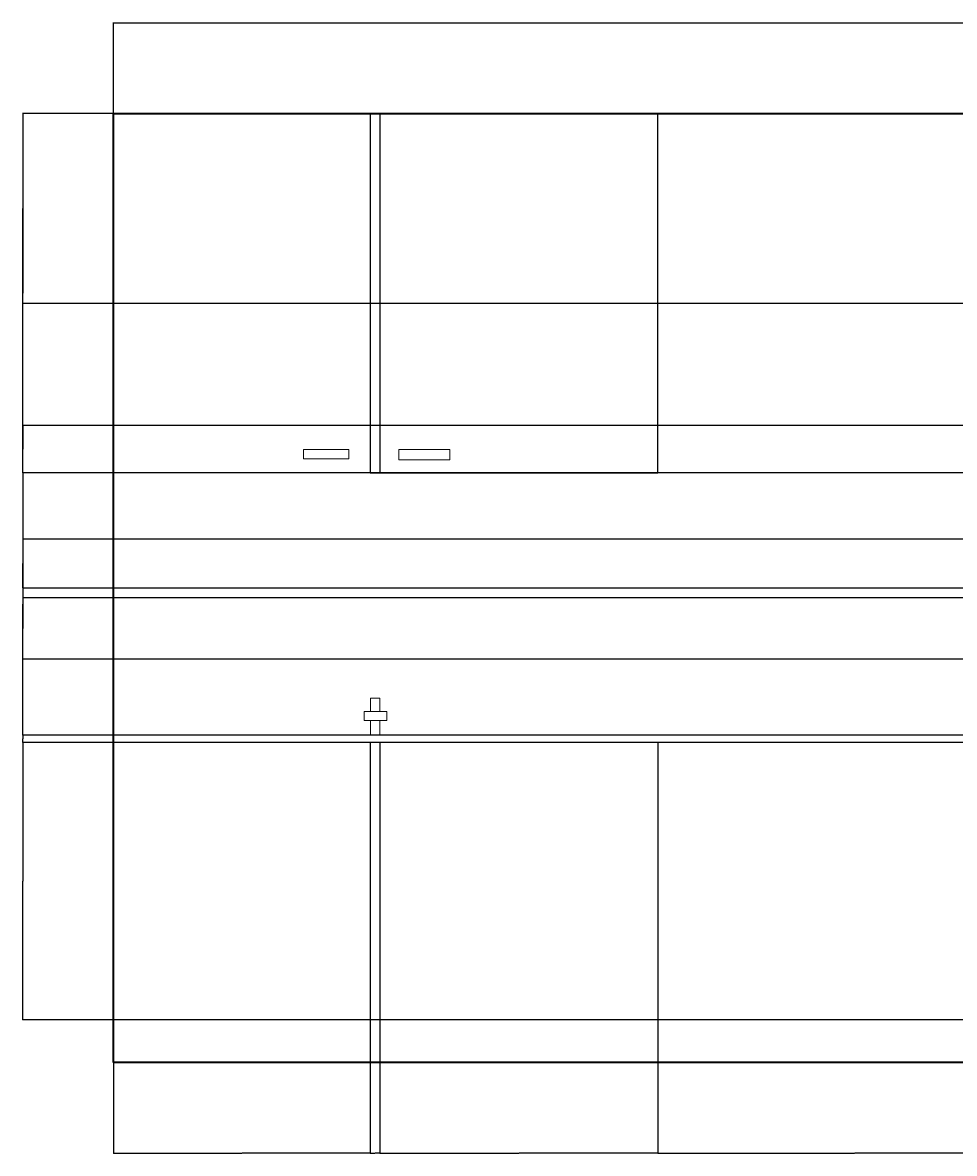
# Model space of a CAD drawing. Units: millimetres. Extents: x 4725 to 8727, y 2935 to 5260.
# Tile 1 of 3: x 4725 to 6642, y 2935 to 5260. Entities that reach past the tile are written whole.
import ezdxf

# ---------------------------------------------------------------- set-up
doc = ezdxf.new("R2010")
doc.units = ezdxf.units.MM
for name, color, linetype, lineweight in [('A-ANNO-DIMS', 2, 'Continuous', 18), ('A-CASE-CTOP', 7, 'Continuous', 25), ('A-CASE-HRDW', 9, 'Continuous', 13), ('A-ELEV', 7, 'Continuous', 35), ('A-FLOR-CASE', 8, 'Continuous', 25), ('A-FLOR-FIXT', 9, 'Continuous', 18)]:
    doc.layers.add(name, color=color, linetype=linetype, lineweight=lineweight)
doc.styles.get("Standard").update_dxf_attribs({"font": 'arial.ttf'})
doc.dimstyles.get("Standard").update_dxf_attribs({"dimtxt": 0.18, "dimasz": 0.18, "dimexe": 0.18, "dimexo": 0.0625, "dimgap": 0.09, "dimtad": 0, "dimtih": 1, "dimtoh": 1, "dimdec": 4, "dimzin": 0, "dimdsep": 46, "dimtxsty": 'Standard', "dimcen": 0.09, "dimadec": 0, "dimazin": 0, "dimtfac": 1, "dimtdec": 4, "dimtofl": 0, "dimtmove": 0, "dimatfit": 3, "dimfxl": 1, "dimtolj": 1, "dimtzin": 0, "dimarcsym": 0})

# ---------------------------------------------------------------- blocks, each defined once
blk = doc.blocks.new('*D7')
at = {"layer": 'A-ANNO-DIMS', "color": 0, "lineweight": -2, "transparency": 16777216}
for p, q in [((4912.4, 3209), (4912.4, 2934.7)), ((5440.1, 3209), (5440.1, 2934.7)), ((4912.5, 2934.8), (5175.9, 2934.8)), ((5440, 2934.8), (5176.6, 2934.8))]:
    blk.add_line(p, q, dxfattribs=at)
at = {"layer": 'A-ANNO-DIMS', "color": 0, "transparency": 16777216}
for points in [[(4912.5, 2934.9), (4912.5, 2934.8), (4912.4, 2934.8)], [(5440, 2934.9), (5440, 2934.8), (5440.1, 2934.8)]]:
    blk.add_solid(points, dxfattribs=at)
at = {"layer": 'Defpoints', "color": 0, "transparency": 16777216}
for p in [(4912.4, 3209), (5440.1, 3209), (5440.1, 2934.8)]:
    blk.add_point(p, dxfattribs=at)
at = {"layer": 'A-ANNO-DIMS', "color": 0, "transparency": 16777216, "insert": (5176.3, 2934.8), "char_height": 0.18, "attachment_point": 5}
blk.add_mtext('\\A1;527.8', dxfattribs=at)
blk = doc.blocks.new('*D8')
at = {"layer": 'A-ANNO-DIMS', "color": 0, "lineweight": -2, "transparency": 16777216}
for p, q in [((5440.1, 3209), (5440.1, 2934.7)), ((5460.1, 3209), (5460.1, 2934.7)), ((5440.3, 2934.8), (5449.9, 2934.8)), ((5460, 2934.8), (5450.4, 2934.8))]:
    blk.add_line(p, q, dxfattribs=at)
at = {"layer": 'A-ANNO-DIMS', "color": 0, "transparency": 16777216}
for points in [[(5440.3, 2934.9), (5440.3, 2934.8), (5440.1, 2934.8)], [(5460, 2934.9), (5460, 2934.8), (5460.1, 2934.8)]]:
    blk.add_solid(points, dxfattribs=at)
at = {"layer": 'Defpoints', "color": 0, "transparency": 16777216}
for p in [(5440.1, 3209), (5460.1, 3209), (5460.1, 2934.8)]:
    blk.add_point(p, dxfattribs=at)
at = {"layer": 'A-ANNO-DIMS', "color": 0, "transparency": 16777216, "insert": (5450.1, 2934.8), "char_height": 0.18, "attachment_point": 5}
blk.add_mtext('\\A1;20', dxfattribs=at)
blk = doc.blocks.new('*D9')
at = {"layer": 'A-ANNO-DIMS', "color": 0, "lineweight": -2, "transparency": 16777216}
for p, q in [((5460.1, 3209), (5460.1, 2934.7)), ((6031.8, 3209), (6031.8, 2934.7)), ((5460.3, 2934.8), (5745.6, 2934.8)), ((6031.6, 2934.8), (5746.4, 2934.8))]:
    blk.add_line(p, q, dxfattribs=at)
at = {"layer": 'A-ANNO-DIMS', "color": 0, "transparency": 16777216}
for points in [[(5460.3, 2934.9), (5460.3, 2934.8), (5460.1, 2934.8)], [(6031.6, 2934.9), (6031.6, 2934.8), (6031.8, 2934.8)]]:
    blk.add_solid(points, dxfattribs=at)
at = {"layer": 'Defpoints', "color": 0, "transparency": 16777216}
for p in [(5460.1, 3209), (6031.8, 3209), (6031.8, 2934.8)]:
    blk.add_point(p, dxfattribs=at)
at = {"layer": 'A-ANNO-DIMS', "color": 0, "transparency": 16777216, "insert": (5746, 2934.8), "char_height": 0.18, "attachment_point": 5}
blk.add_mtext('\\A1;571.6', dxfattribs=at)
blk = doc.blocks.new('*D10')
at = {"layer": 'A-ANNO-DIMS', "color": 0, "lineweight": -2, "transparency": 16777216}
for p, q in [((6031.8, 3209), (6031.8, 2934.7)), ((6841.9, 3209), (6841.9, 2934.7)), ((6032, 2934.8), (6436.5, 2934.8)), ((6841.8, 2934.8), (6437.3, 2934.8))]:
    blk.add_line(p, q, dxfattribs=at)
at = {"layer": 'A-ANNO-DIMS', "color": 0, "transparency": 16777216}
for points in [[(6032, 2934.9), (6032, 2934.8), (6031.8, 2934.8)], [(6841.8, 2934.9), (6841.8, 2934.8), (6841.9, 2934.8)]]:
    blk.add_solid(points, dxfattribs=at)
at = {"layer": 'Defpoints', "color": 0, "transparency": 16777216}
for p in [(6031.8, 3209), (6841.9, 3209), (6841.9, 2934.8)]:
    blk.add_point(p, dxfattribs=at)
at = {"layer": 'A-ANNO-DIMS', "color": 0, "transparency": 16777216, "insert": (6436.9, 2934.8), "char_height": 0.18, "attachment_point": 5}
blk.add_mtext('\\A1;810.2', dxfattribs=at)
blk = doc.blocks.new('*D22')
at = {"layer": 'A-ANNO-DIMS', "color": 0, "lineweight": -2, "transparency": 16777216}
for p, q in [((4912.3, 3779.7), (4725.3, 3779.7)), ((4725.5, 3779.5), (4725.5, 3494.5)), ((4725.5, 3209.2), (4725.5, 3494.2)), ((4912.3, 3209), (4725.3, 3209))]:
    blk.add_line(p, q, dxfattribs=at)
at = {"layer": 'A-ANNO-DIMS', "color": 0, "transparency": 16777216}
for points in [[(4725.5, 3779.5), (4725.5, 3779.5), (4725.5, 3779.7)], [(4725.5, 3209.2), (4725.5, 3209.2), (4725.5, 3209)]]:
    blk.add_solid(points, dxfattribs=at)
at = {"layer": 'Defpoints', "color": 0, "transparency": 16777216}
for p in [(4725.5, 3779.7), (4912.4, 3779.7), (4912.4, 3209)]:
    blk.add_point(p, dxfattribs=at)
at = {"layer": 'A-ANNO-DIMS', "color": 0, "transparency": 16777216, "insert": (4725.5, 3494.4), "char_height": 0.18, "attachment_point": 5}
blk.add_mtext('\\A1;570.7', dxfattribs=at)
blk = doc.blocks.new('*D23')
at = {"layer": 'A-ANNO-DIMS', "color": 0, "lineweight": -2, "transparency": 16777216}
for p, q in [((4912.3, 3794.7), (4725.3, 3794.7)), ((4725.5, 3794.5), (4725.5, 3787.4)), ((4912.3, 3779.7), (4725.3, 3779.7)), ((4725.5, 3779.9), (4725.5, 3787))]:
    blk.add_line(p, q, dxfattribs=at)
at = {"layer": 'A-ANNO-DIMS', "color": 0, "transparency": 16777216}
for points in [[(4725.5, 3794.5), (4725.5, 3794.5), (4725.5, 3794.7)], [(4725.5, 3779.9), (4725.5, 3779.9), (4725.5, 3779.7)]]:
    blk.add_solid(points, dxfattribs=at)
at = {"layer": 'Defpoints', "color": 0, "transparency": 16777216}
for p in [(4725.5, 3794.7), (4912.4, 3794.7), (4912.4, 3779.7)]:
    blk.add_point(p, dxfattribs=at)
at = {"layer": 'A-ANNO-DIMS', "color": 0, "transparency": 16777216, "insert": (4725.5, 3787.2), "char_height": 0.18, "attachment_point": 5}
blk.add_mtext('\\A1;15', dxfattribs=at)
blk = doc.blocks.new('*D24')
at = {"layer": 'A-ANNO-DIMS', "color": 0, "lineweight": -2, "transparency": 16777216}
for p, q in [((4912.3, 4334.2), (4725.3, 4334.2)), ((4725.5, 4334), (4725.5, 4064.6)), ((4725.5, 3794.9), (4725.5, 4064.3)), ((4912.3, 3794.7), (4725.3, 3794.7))]:
    blk.add_line(p, q, dxfattribs=at)
at = {"layer": 'A-ANNO-DIMS', "color": 0, "transparency": 16777216}
for points in [[(4725.5, 4334), (4725.5, 4334), (4725.5, 4334.2)], [(4725.5, 3794.9), (4725.5, 3794.9), (4725.5, 3794.7)]]:
    blk.add_solid(points, dxfattribs=at)
at = {"layer": 'Defpoints', "color": 0, "transparency": 16777216}
for p in [(4725.5, 4334.2), (4912.4, 4334.2), (4912.4, 3794.7)]:
    blk.add_point(p, dxfattribs=at)
at = {"layer": 'A-ANNO-DIMS', "color": 0, "transparency": 16777216, "insert": (4725.5, 4064.5), "char_height": 0.18, "attachment_point": 5}
blk.add_mtext('\\A1;539.5', dxfattribs=at)
blk = doc.blocks.new('*D25')
at = {"layer": 'A-ANNO-DIMS', "color": 0, "lineweight": -2, "transparency": 16777216}
for p, q in [((4912.3, 5073.1), (4725.3, 5073.1)), ((4725.5, 5072.9), (4725.5, 4703.8)), ((4725.5, 4334.4), (4725.5, 4703.5)), ((4912.3, 4334.2), (4725.3, 4334.2))]:
    blk.add_line(p, q, dxfattribs=at)
at = {"layer": 'A-ANNO-DIMS', "color": 0, "transparency": 16777216}
for points in [[(4725.5, 5072.9), (4725.5, 5072.9), (4725.5, 5073.1)], [(4725.5, 4334.4), (4725.5, 4334.4), (4725.5, 4334.2)]]:
    blk.add_solid(points, dxfattribs=at)
at = {"layer": 'Defpoints', "color": 0, "transparency": 16777216}
for p in [(4725.5, 5073.1), (4912.4, 5073.1), (4912.4, 4334.2)]:
    blk.add_point(p, dxfattribs=at)
at = {"layer": 'A-ANNO-DIMS', "color": 0, "transparency": 16777216, "insert": (4725.5, 4703.7), "char_height": 0.18, "attachment_point": 5}
blk.add_mtext('\\A1;738.9', dxfattribs=at)
blk = doc.blocks.new('*D30')
at = {"layer": 'A-ANNO-DIMS', "color": 0, "lineweight": -2, "transparency": 16777216}
for p, q in [((8205.1, 5073.1), (4725.3, 5073.1)), ((4725.5, 5072.9), (4725.5, 4878)), ((4725.5, 4682.6), (4725.5, 4877.6)), ((7900.8, 4682.5), (4725.3, 4682.5))]:
    blk.add_line(p, q, dxfattribs=at)
at = {"layer": 'A-ANNO-DIMS', "color": 0, "transparency": 16777216}
for points in [[(4725.5, 5072.9), (4725.5, 5072.9), (4725.5, 5073.1)], [(4725.5, 4682.6), (4725.5, 4682.6), (4725.5, 4682.5)]]:
    blk.add_solid(points, dxfattribs=at)
at = {"layer": 'Defpoints', "color": 0, "transparency": 16777216}
for p in [(4725.5, 5073.1), (8205.2, 5073.1), (7900.9, 4682.5)]:
    blk.add_point(p, dxfattribs=at)
at = {"layer": 'A-ANNO-DIMS', "color": 0, "transparency": 16777216, "insert": (4725.5, 4877.8), "char_height": 0.18, "attachment_point": 5}
blk.add_mtext('\\A1;390.7', dxfattribs=at)
blk = doc.blocks.new('*D31')
at = {"layer": 'A-ANNO-DIMS', "color": 0, "lineweight": -2, "transparency": 16777216}
for p, q in [((6841.9, 4431.6), (4725.3, 4431.6)), ((4725.5, 4431.4), (4725.5, 4383.1)), ((4725.5, 4334.4), (4725.5, 4382.7)), ((6841.9, 4334.2), (4725.3, 4334.2))]:
    blk.add_line(p, q, dxfattribs=at)
at = {"layer": 'A-ANNO-DIMS', "color": 0, "transparency": 16777216}
for points in [[(4725.5, 4431.4), (4725.5, 4431.4), (4725.5, 4431.6)], [(4725.5, 4334.4), (4725.5, 4334.4), (4725.5, 4334.2)]]:
    blk.add_solid(points, dxfattribs=at)
at = {"layer": 'Defpoints', "color": 0, "transparency": 16777216}
for p in [(4725.5, 4431.6), (6841.9, 4431.6), (6841.9, 4334.2)]:
    blk.add_point(p, dxfattribs=at)
at = {"layer": 'A-ANNO-DIMS', "color": 0, "transparency": 16777216, "insert": (4725.5, 4382.9), "char_height": 0.18, "attachment_point": 5}
blk.add_mtext('\\A1;97.4', dxfattribs=at)
blk = doc.blocks.new('*D40')
at = {"layer": 'A-ANNO-DIMS', "color": 0, "lineweight": -2, "transparency": 16777216}
for p, q in [((4912.4, 5073.2), (4912.4, 5260.1)), ((4912.5, 5260), (6725.6, 5260)), ((8539.4, 5260), (6726.3, 5260)), ((8539.6, 5073.2), (8539.6, 5260.1))]:
    blk.add_line(p, q, dxfattribs=at)
at = {"layer": 'A-ANNO-DIMS', "color": 0, "transparency": 16777216}
for points in [[(4912.5, 5260), (4912.5, 5259.9), (4912.4, 5260)], [(8539.4, 5260), (8539.4, 5259.9), (8539.6, 5260)]]:
    blk.add_solid(points, dxfattribs=at)
at = {"layer": 'Defpoints', "color": 0, "transparency": 16777216}
for p in [(8539.6, 5260), (4912.4, 5073.1), (8539.6, 5073.1)]:
    blk.add_point(p, dxfattribs=at)
at = {"layer": 'A-ANNO-DIMS', "color": 0, "transparency": 16777216, "insert": (6726, 5260), "char_height": 0.18, "attachment_point": 5}
blk.add_mtext('\\A1;3627', dxfattribs=at)
blk = doc.blocks.new('*D41')
at = {"layer": 'A-ANNO-DIMS', "color": 0, "lineweight": -2, "transparency": 16777216}
for p, q in [((4912.4, 5073.1), (8726.6, 5073.1)), ((8726.4, 5072.9), (8726.4, 4097.6)), ((8726.4, 3121.9), (8726.4, 4097.2)), ((8539.6, 3121.7), (8726.6, 3121.7))]:
    blk.add_line(p, q, dxfattribs=at)
at = {"layer": 'A-ANNO-DIMS', "color": 0, "transparency": 16777216}
for points in [[(8726.4, 5072.9), (8726.4, 5072.9), (8726.4, 5073.1)], [(8726.4, 3121.9), (8726.4, 3121.9), (8726.4, 3121.7)]]:
    blk.add_solid(points, dxfattribs=at)
at = {"layer": 'Defpoints', "color": 0, "transparency": 16777216}
for p in [(4912.4, 5073.1), (8726.4, 5073.1), (8539.6, 3121.7)]:
    blk.add_point(p, dxfattribs=at)
at = {"layer": 'A-ANNO-DIMS', "color": 0, "transparency": 16777216, "insert": (8726.4, 4097.4), "char_height": 0.18, "attachment_point": 5}
blk.add_mtext('\\A1;1951.4', dxfattribs=at)
blk = doc.blocks.new('*D42')
at = {"layer": 'A-ANNO-DIMS', "color": 0, "lineweight": -2, "transparency": 16777216}
for p, q in [((7900.8, 4077.4), (4725.3, 4077.4)), ((4725.5, 4077.2), (4725.5, 4014.3)), ((4725.5, 3951), (4725.5, 4013.9)), ((7969.7, 3950.8), (4725.3, 3950.8))]:
    blk.add_line(p, q, dxfattribs=at)
at = {"layer": 'A-ANNO-DIMS', "color": 0, "transparency": 16777216}
for points in [[(4725.5, 4077.2), (4725.5, 4077.2), (4725.5, 4077.4)], [(4725.5, 3951), (4725.5, 3951), (4725.5, 3950.8)]]:
    blk.add_solid(points, dxfattribs=at)
at = {"layer": 'Defpoints', "color": 0, "transparency": 16777216}
for p in [(7900.9, 4077.4), (4725.5, 3950.8), (7969.8, 3950.8)]:
    blk.add_point(p, dxfattribs=at)
at = {"layer": 'A-ANNO-DIMS', "color": 0, "transparency": 16777216, "insert": (4725.5, 4014.1), "char_height": 0.18, "attachment_point": 5}
blk.add_mtext('\\A1;126.6', dxfattribs=at)
blk = doc.blocks.new('*D43')
at = {"layer": 'A-ANNO-DIMS', "color": 0, "lineweight": -2, "transparency": 16777216}
for p, q in [((7969.7, 4198), (4725.3, 4198)), ((4725.5, 4197.8), (4725.5, 4147.9)), ((4725.5, 4097.6), (4725.5, 4147.5)), ((7900.8, 4097.4), (4725.3, 4097.4))]:
    blk.add_line(p, q, dxfattribs=at)
at = {"layer": 'A-ANNO-DIMS', "color": 0, "transparency": 16777216}
for points in [[(4725.5, 4197.8), (4725.5, 4197.8), (4725.5, 4198)], [(4725.5, 4097.6), (4725.5, 4097.6), (4725.5, 4097.4)]]:
    blk.add_solid(points, dxfattribs=at)
at = {"layer": 'Defpoints', "color": 0, "transparency": 16777216}
for p in [(4725.5, 4198), (7969.8, 4198), (7900.9, 4097.4)]:
    blk.add_point(p, dxfattribs=at)
at = {"layer": 'A-ANNO-DIMS', "color": 0, "transparency": 16777216, "insert": (4725.5, 4147.7), "char_height": 0.18, "attachment_point": 5}
blk.add_mtext('\\A1;100.6', dxfattribs=at)

msp = doc.modelspace()

# ---------------------------------------------------------------- linework, layer by layer
at = {"layer": 'A-CASE-CTOP'}
for p, q in [((7900.8562, 3794.7145), (4912.3658, 3794.7145)), ((7900.8562, 3779.7145), (4912.3658, 3779.7145))]:
    msp.add_line(p, q, dxfattribs=at)
at = {"layer": 'A-CASE-HRDW'}
for points in [[(5396.4714, 4382.2166), (5303.3102, 4382.2166), (5303.3102, 4362.9052), (5396.4714, 4362.9052)], [(5499.0535, 4382.2166), (5603.9647, 4382.2166), (5603.9647, 4361.2524), (5499.0535, 4361.2524)]]:
    msp.add_lwpolyline(points, close=True, dxfattribs=at)
at = {"layer": 'A-ELEV'}
for p, q in [((4912.3658, 5073.1177), (8539.5662, 5073.1177)), ((4912.3658, 3121.6884), (4912.3658, 5073.1177)), ((8539.5662, 3121.6884), (4912.3658, 3121.6884))]:
    msp.add_line(p, q, dxfattribs=at)
at = {"layer": 'A-FLOR-CASE'}
for p, q in [((5440.142, 5073.1177), (5440.142, 4334.1944)), ((5460.142, 5073.1177), (5460.142, 4334.1944)), ((6031.7891, 4334.1944), (6031.7891, 5073.1177)), ((6031.7891, 5073.1177), (6841.9423, 5073.1177)), ((5440.142, 4334.1944), (4912.3658, 4334.1944)), ((5440.142, 4334.1944), (5460.142, 4334.1944)), ((5460.142, 4334.1944), (6031.7891, 4334.1944)), ((6841.9423, 4334.1944), (6031.7891, 4334.1944)), ((5440.142, 3779.7145), (5440.142, 3209.0157)), ((5460.142, 3779.7145), (5460.142, 3209.0157)), ((8539.5662, 3209.0157), (4912.3658, 3209.0157))]:
    msp.add_line(p, q, dxfattribs=at)
msp.add_lwpolyline([(6031.7891, 3779.7145), (6031.7891, 3209.0157)], dxfattribs=at)
at = {"layer": 'A-FLOR-FIXT'}
for p, q in [((5440.8131, 3843.1564), (5440.8131, 3870.909)), ((5440.8131, 3870.909), (5460.142, 3870.909)), ((5460.142, 3870.909), (5460.142, 3843.1564)), ((5440.8131, 3794.7145), (5440.8131, 3825.1403)), ((5440.8131, 3825.1403), (5460.142, 3825.1403)), ((5460.142, 3825.1403), (5460.142, 3794.7145))]:
    msp.add_line(p, q, dxfattribs=at)
msp.add_lwpolyline([(5427.9046, 3843.1564), (5474.1987, 3843.1564), (5474.1987, 3825.1403), (5427.9046, 3825.1403)], close=True, dxfattribs=at)

# ---------------------------------------------------------------- dimensions: what is measured, and where the dimension line sits
at = {"layer": 'A-ANNO-DIMS'}
for base, p1, p2, override, picture, middle in [((8539.5662, 5259.9677), (4912.3658, 5073.1177), (8539.5662, 5073.1177), {"dimdec": 0, "dimlfac": 1, "dimrnd": 0, "dimzin": 0, "dimdsep": 46, "dimlunit": 2}, '*D40', (6725.966, 5259.9677)), ((5440.142, 2934.8384), (4912.3658, 3209.0157), (5440.142, 3209.0157), {"dimdec": 1, "dimlfac": 1, "dimrnd": 0, "dimzin": 0, "dimdsep": 46, "dimlunit": 2}, '*D7', (5176.2539, 2934.8384)), ((5460.142, 2934.8384), (5440.142, 3209.0157), (5460.142, 3209.0157), {"dimdec": 0, "dimlfac": 1, "dimrnd": 0, "dimzin": 0, "dimdsep": 46, "dimlunit": 2}, '*D8', (5450.142, 2934.8384)), ((6031.7891, 2934.8384), (5460.142, 3209.0157), (6031.7891, 3209.0157), {"dimdec": 1, "dimlfac": 1, "dimrnd": 0, "dimzin": 0, "dimdsep": 46, "dimlunit": 2}, '*D9', (5745.9655, 2934.8384)), ((6841.9423, 2934.8384), (6031.7891, 3209.0157), (6841.9423, 3209.0157), {"dimdec": 1, "dimlfac": 1, "dimrnd": 0, "dimzin": 0, "dimdsep": 46, "dimlunit": 2}, '*D10', (6436.8657, 2934.8384))]:
    dim = msp.add_linear_dim(base=base, p1=p1, p2=p2, dimstyle='Standard', override=override, dxfattribs=at)
    dim.commit()
    dim.dimension.update_dxf_attribs({"geometry": picture, "text_midpoint": middle})
for base, p1, p2, override, picture, middle in [((4725.5158, 5073.1177), (4912.3658, 4334.1944), (4912.3658, 5073.1177), {"dimdec": 1, "dimlfac": 1, "dimrnd": 0, "dimzin": 0, "dimdsep": 46, "dimlunit": 2}, '*D25', (4725.5158, 4703.6561)), ((4725.5158, 5073.1177), (7900.8562, 4682.4503), (8205.2112, 5073.1177), {"dimdec": 1, "dimlfac": 1, "dimrnd": 0, "dimzin": 0, "dimdsep": 46, "dimlunit": 2}, '*D30', (4725.5158, 4877.784)), ((8726.4162, 5073.1177), (8539.5662, 3121.6884), (4912.3658, 5073.1177), {"dimdec": 1, "dimlfac": 1, "dimrnd": 0, "dimzin": 0, "dimdsep": 46, "dimlunit": 2}, '*D41', (8726.4162, 4097.4031)), ((4725.5158, 4431.5979), (6841.9423, 4334.1944), (6841.9423, 4431.5979), {"dimdec": 1, "dimlfac": 1, "dimrnd": 0, "dimzin": 0, "dimdsep": 46, "dimlunit": 2}, '*D31', (4725.5158, 4382.8962)), ((4725.5158, 4334.1944), (4912.3658, 3794.7145), (4912.3658, 4334.1944), {"dimdec": 1, "dimlfac": 1, "dimrnd": 0, "dimzin": 0, "dimdsep": 46, "dimlunit": 2}, '*D24', (4725.5158, 4064.4545)), ((4725.5158, 4197.9992), (7900.8562, 4097.4031), (7969.7678, 4197.9992), {"dimdec": 1, "dimlfac": 1, "dimrnd": 0, "dimzin": 0, "dimdsep": 46, "dimlunit": 2}, '*D43', (4725.5158, 4147.7011)), ((4725.5158, 3950.7955), (7900.8562, 4077.4031), (7969.7678, 3950.7955), {"dimdec": 1, "dimlfac": 1, "dimrnd": 0, "dimzin": 0, "dimdsep": 46, "dimlunit": 2}, '*D42', (4725.5158, 4014.0993)), ((4725.5158, 3794.7145), (4912.3658, 3779.7145), (4912.3658, 3794.7145), {"dimdec": 0, "dimlfac": 1, "dimrnd": 0, "dimzin": 0, "dimdsep": 46, "dimlunit": 2}, '*D23', (4725.5158, 3787.2145)), ((4725.5158, 3779.7145), (4912.3658, 3209.0157), (4912.3658, 3779.7145), {"dimdec": 1, "dimlfac": 1, "dimrnd": 0, "dimzin": 0, "dimdsep": 46, "dimlunit": 2}, '*D22', (4725.5158, 3494.3651))]:
    dim = msp.add_linear_dim(base=base, p1=p1, p2=p2, angle=90, dimstyle='Standard', override=override, dxfattribs=at)
    dim.commit()
    dim.dimension.update_dxf_attribs({"geometry": picture, "text_midpoint": middle})

doc.saveas('drawing.dxf')
